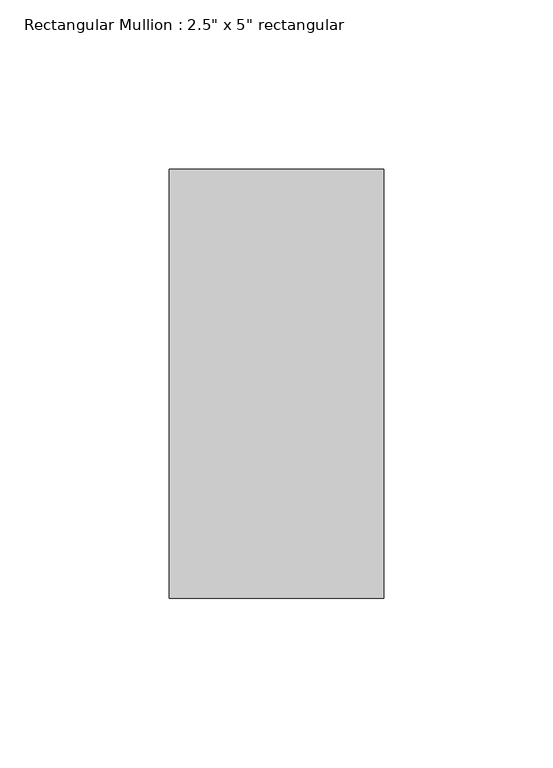
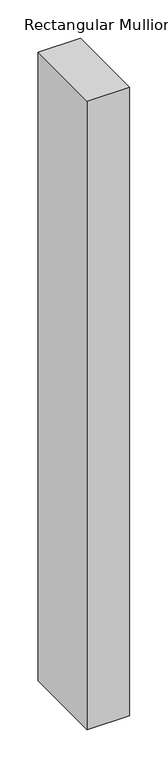
"""IFC4 building model written with IfcOpenShell, lengths in millimetres: member geometry."""

from ifc_helpers import new_model, si_unit, frame, origin, place, context, project, spatial, polyline, outline, extrude, source, transform, mapped, element, save


def member_883d71fc(model_context):
    return source(origin(), model_context, "Body", "SweptSolid", [
        extrude(outline(polyline([(0.0, 63.5), (0.0, -63.5), (-63.5, -63.5), (-63.5, 63.5), (0.0, 63.5)])), frame((0.0, 0.0, -996.95), z_axis=(0.0, 0.0, 1.0), x_axis=(1.0, 0.0, 0.0)), (0.0, 0.0, 1.0), 996.95),
    ])


if __name__ == "__main__":
    model = new_model("IFC4")
    model_context = context("Model", 3, world=origin())
    ifc_project = project(units=[si_unit("LENGTHUNIT", "METRE", prefix="MILLI")], contexts=[model_context])
    site = spatial("IfcSite", under=ifc_project)
    building = spatial("IfcBuilding", under=site)
    placement = place(None, origin())
    member_shape = member_883d71fc(model_context)
    element("IfcMember", 1, ObjectType="Rectangular Mullion : 2.5\" x 5\" rectangular", at=placement, inside=building, context=model_context, shape_type="MappedRepresentation", body=[
        mapped(member_shape, transform((0.0, 0.0, 0.0), x_axis=(1.0, 0.0, 0.0), y_axis=(0.0, 1.0, 0.0), z_axis=(0.0, 0.0, 1.0))),
    ])
    save(model, "model.ifc")

# Revit data of these elements
# Type "Rectangular Mullion : 2.5\" x 5\" rectangular"
#   built-in parameter 1007304 = 0.416667 (stored number, unit not read)
#   built-in parameter 1007301 = 0.104167 (stored number, unit not read)
#   built-in parameter 1007300 = 0.104167 (stored number, unit not read)
# Element 1 (IfcMember, "Rectangular Mullion : 2.5\" x 5\" rectangular")
#   Materials on its faces: "Aluminum"
# Materials
#   "Aluminum": class "Metal", colour RGB 247 247 247, transparency 0, Description = "Aluminum 6061", Cost = 0
